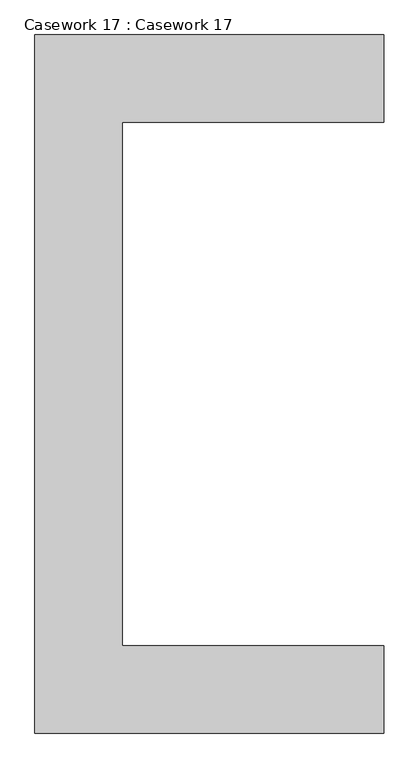
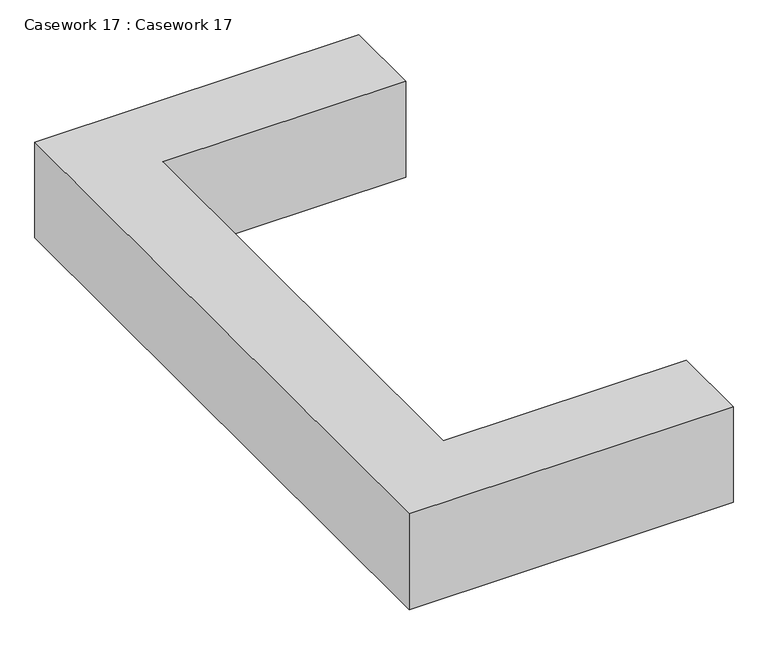
"""IFC4 building model written with IfcOpenShell, lengths in millimetres: furniture geometry, Casework 17 : Casework 17."""

from ifc_helpers import new_model, si_unit, frame, origin, place, context, project, spatial, polyline, outline, extrude, source, transform, mapped, element, save


def casework_17_casework_17_2f46c277(model_context):
    return source(origin(), model_context, "Body", "SweptSolid", [
        extrude(outline(polyline([(-14339.1107921, -3694.8987034), (-11939.1107921, -3694.8987034), (-11939.1107921, -4294.8987034), (-13739.1107921, -4294.8987034), (-13739.1107921, -7894.8987034), (-11939.1107921, -7894.8987034), (-11939.1107921, -8494.8987034), (-14339.1107921, -8494.8987034), (-14339.1107921, -3694.8987034)])), frame((0.0, 0.0, 600.0), z_axis=(0.0, 0.0, 1.0), x_axis=(1.0, 0.0, 0.0)), (0.0, 0.0, 1.0), 750.0),
    ])


if __name__ == "__main__":
    model = new_model("IFC4")
    model_context = context("Model", 3, world=origin())
    ifc_project = project(units=[si_unit("LENGTHUNIT", "METRE", prefix="MILLI")], contexts=[model_context])
    site = spatial("IfcSite", under=ifc_project)
    building = spatial("IfcBuilding", under=site)
    placement = place(None, origin())
    casework_17_casework_17_shape = casework_17_casework_17_2f46c277(model_context)
    element("IfcFurniture", 1, ObjectType="Casework 17 : Casework 17", at=placement, inside=building, context=model_context, shape_type="MappedRepresentation", body=[
        mapped(casework_17_casework_17_shape, transform((0.0, 0.0, 0.0), x_axis=(1.0, 0.0, 0.0), y_axis=(0.0, 1.0, 0.0), z_axis=(0.0, 0.0, 1.0))),
    ])
    save(model, "model.ifc")

# Revit data of these elements
# Element 1 (IfcFurniture, "Casework 17 : Casework 17")
#   Materials on its faces: "MY KITCHEN CABINET"
# Materials
#   "MY KITCHEN CABINET": class "Metal", colour RGB 200 200 200, transparency 0, Description = "Aluminum 6061", Cost = 0
